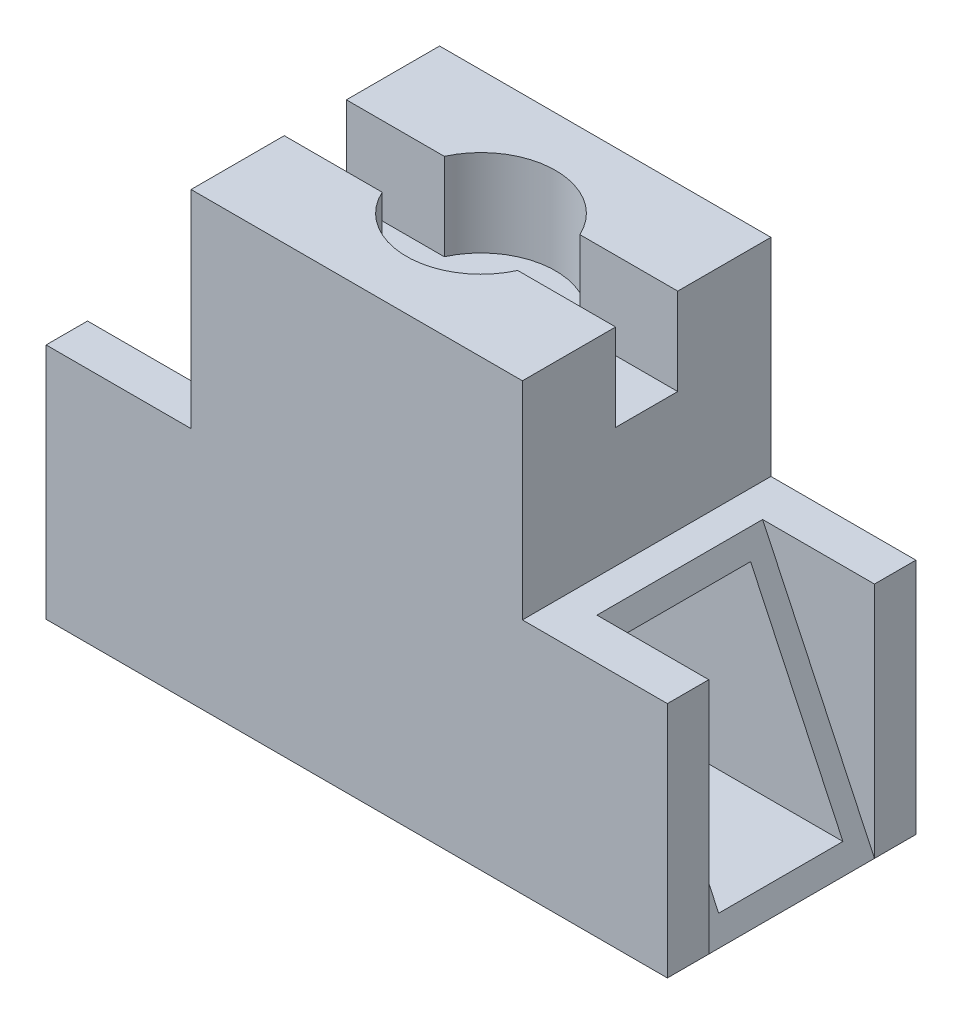
ISO-10303-21;
HEADER;
FILE_DESCRIPTION(('STEP AP214'),'2;1');
FILE_NAME('part.step','',(''),(''),'','','');
FILE_SCHEMA(('AUTOMOTIVE_DESIGN { 1 0 10303 214 1 1 1 1 }'));
ENDSEC;
DATA;
#1=APPLICATION_CONTEXT('core data for automotive mechanical design processes');
#2=APPLICATION_PROTOCOL_DEFINITION('international standard','automotive_design',2000,#1);
#3=PRODUCT_CONTEXT('',#1,'mechanical');
#4=PRODUCT('Part','Part','',(#3));
#5=PRODUCT_RELATED_PRODUCT_CATEGORY('part','',(#4));
#6=PRODUCT_DEFINITION_FORMATION('','',#4);
#7=PRODUCT_DEFINITION_CONTEXT('part definition',#1,'design');
#8=PRODUCT_DEFINITION('design','',#6,#7);
#9=PRODUCT_DEFINITION_SHAPE('','',#8);
#10=(LENGTH_UNIT() NAMED_UNIT(*) SI_UNIT(.MILLI.,.METRE.));
#11=(NAMED_UNIT(*) PLANE_ANGLE_UNIT() SI_UNIT($,.RADIAN.));
#12=(NAMED_UNIT(*) SI_UNIT($,.STERADIAN.) SOLID_ANGLE_UNIT());
#13=UNCERTAINTY_MEASURE_WITH_UNIT(LENGTH_MEASURE(1.E-05),#10,'distance_accuracy_value','');
#14=(GEOMETRIC_REPRESENTATION_CONTEXT(3) GLOBAL_UNCERTAINTY_ASSIGNED_CONTEXT((#13)) GLOBAL_UNIT_ASSIGNED_CONTEXT((#10,
#11,#12)) REPRESENTATION_CONTEXT('',''));
#15=CARTESIAN_POINT('',(0.,0.,0.));
#16=DIRECTION('',(0.,0.,1.));
#17=DIRECTION('',(1.,0.,0.));
#18=AXIS2_PLACEMENT_3D('',#15,#16,#17);
#19=CARTESIAN_POINT('',(75.,28.6870588235294,-60.));
#20=DIRECTION('',(1.,0.,0.));
#21=DIRECTION('',(0.,0.,-1.));
#22=AXIS2_PLACEMENT_3D('',#19,#20,#21);
#23=PLANE('',#22);
#24=DIRECTION('',(0.,0.,1.));
#25=VECTOR('',#24,1.);
#26=CARTESIAN_POINT('',(75.,-28.6870588235294,-60.));
#27=LINE('',#26,#25);
#28=CARTESIAN_POINT('',(75.,-28.6870588235294,-10.));
#29=VERTEX_POINT('',#28);
#30=CARTESIAN_POINT('',(75.,-28.6870588235294,0.));
#31=VERTEX_POINT('',#30);
#32=EDGE_CURVE('E257',#29,#31,#27,.T.);
#33=ORIENTED_EDGE('',*,*,#32,.F.);
#34=DIRECTION('',(0.,1.,0.));
#35=VECTOR('',#34,1.);
#36=CARTESIAN_POINT('',(75.,-28.6870588235294,-10.));
#37=LINE('',#36,#35);
#38=CARTESIAN_POINT('',(75.,28.6870588235294,-10.));
#39=VERTEX_POINT('',#38);
#40=EDGE_CURVE('E399',#29,#39,#37,.T.);
#41=ORIENTED_EDGE('',*,*,#40,.T.);
#42=DIRECTION('',(0.,0.,1.));
#43=VECTOR('',#42,1.);
#44=CARTESIAN_POINT('',(75.,28.6870588235294,-60.));
#45=LINE('',#44,#43);
#46=CARTESIAN_POINT('',(75.,28.6870588235294,0.));
#47=VERTEX_POINT('',#46);
#48=EDGE_CURVE('E255',#39,#47,#45,.T.);
#49=ORIENTED_EDGE('',*,*,#48,.T.);
#50=DIRECTION('',(0.,1.,0.));
#51=VECTOR('',#50,1.);
#52=CARTESIAN_POINT('',(75.,28.6870588235294,0.));
#53=LINE('',#52,#51);
#54=EDGE_CURVE('E286',#31,#47,#53,.T.);
#55=ORIENTED_EDGE('',*,*,#54,.F.);
#56=EDGE_LOOP('',(#33,#41,#49,#55));
#57=FACE_BOUND('',#56,.T.);
#58=ADVANCED_FACE('F39',(#57),#23,.T.);
#59=CARTESIAN_POINT('',(-75.,28.6870588235294,-60.));
#60=DIRECTION('',(-1.,0.,0.));
#61=DIRECTION('',(0.,0.,1.));
#62=AXIS2_PLACEMENT_3D('',#59,#60,#61);
#63=PLANE('',#62);
#64=DIRECTION('',(0.,0.,1.));
#65=VECTOR('',#64,1.);
#66=CARTESIAN_POINT('',(-75.,28.6870588235294,-60.));
#67=LINE('',#66,#65);
#68=CARTESIAN_POINT('',(-75.,28.6870588235294,-10.));
#69=VERTEX_POINT('',#68);
#70=CARTESIAN_POINT('',(-75.,28.6870588235294,0.));
#71=VERTEX_POINT('',#70);
#72=EDGE_CURVE('E232',#69,#71,#67,.T.);
#73=ORIENTED_EDGE('',*,*,#72,.F.);
#74=DIRECTION('',(0.,-1.,0.));
#75=VECTOR('',#74,1.);
#76=CARTESIAN_POINT('',(-75.,-28.6870588235294,-10.));
#77=LINE('',#76,#75);
#78=CARTESIAN_POINT('',(-75.,-28.6870588235294,-10.));
#79=VERTEX_POINT('',#78);
#80=EDGE_CURVE('E417',#69,#79,#77,.T.);
#81=ORIENTED_EDGE('',*,*,#80,.T.);
#82=DIRECTION('',(0.,0.,1.));
#83=VECTOR('',#82,1.);
#84=CARTESIAN_POINT('',(-75.,-28.6870588235294,-60.));
#85=LINE('',#84,#83);
#86=CARTESIAN_POINT('',(-75.,-28.6870588235294,0.));
#87=VERTEX_POINT('',#86);
#88=EDGE_CURVE('E233',#79,#87,#85,.T.);
#89=ORIENTED_EDGE('',*,*,#88,.T.);
#90=DIRECTION('',(0.,-1.,0.));
#91=VECTOR('',#90,1.);
#92=CARTESIAN_POINT('',(-75.,28.6870588235294,0.));
#93=LINE('',#92,#91);
#94=EDGE_CURVE('E267',#71,#87,#93,.T.);
#95=ORIENTED_EDGE('',*,*,#94,.F.);
#96=EDGE_LOOP('',(#73,#81,#89,#95));
#97=FACE_BOUND('',#96,.T.);
#98=ADVANCED_FACE('F430',(#97),#63,.T.);
#99=CARTESIAN_POINT('',(-75.,28.6870588235294,-60.));
#100=DIRECTION('',(0.,1.,0.));
#101=DIRECTION('',(-1.,0.,0.));
#102=AXIS2_PLACEMENT_3D('',#99,#100,#101);
#103=PLANE('',#102);
#104=DIRECTION('',(0.,0.,1.));
#105=VECTOR('',#104,1.);
#106=CARTESIAN_POINT('',(-48.,28.6870588235294,-50.));
#107=LINE('',#106,#105);
#108=CARTESIAN_POINT('',(-48.,28.6870588235294,-50.));
#109=VERTEX_POINT('',#108);
#110=CARTESIAN_POINT('',(-48.,28.6870588235294,-10.));
#111=VERTEX_POINT('',#110);
#112=EDGE_CURVE('E392',#109,#111,#107,.T.);
#113=ORIENTED_EDGE('',*,*,#112,.T.);
#114=DIRECTION('',(-1.,0.,0.));
#115=VECTOR('',#114,1.);
#116=CARTESIAN_POINT('',(-75.,28.6870588235294,-10.));
#117=LINE('',#116,#115);
#118=EDGE_CURVE('E403',#111,#69,#117,.T.);
#119=ORIENTED_EDGE('',*,*,#118,.T.);
#120=ORIENTED_EDGE('',*,*,#72,.T.);
#121=DIRECTION('',(-1.,0.,0.));
#122=VECTOR('',#121,1.);
#123=CARTESIAN_POINT('',(-75.,28.6870588235294,0.));
#124=LINE('',#123,#122);
#125=CARTESIAN_POINT('',(-40.,28.6870588235294,0.));
#126=VERTEX_POINT('',#125);
#127=EDGE_CURVE('E275',#126,#71,#124,.T.);
#128=ORIENTED_EDGE('',*,*,#127,.F.);
#129=DIRECTION('',(0.,0.,1.));
#130=VECTOR('',#129,1.);
#131=CARTESIAN_POINT('',(-40.,28.6870588235294,-60.));
#132=LINE('',#131,#130);
#133=CARTESIAN_POINT('',(-40.,28.6870588235294,-60.));
#134=VERTEX_POINT('',#133);
#135=EDGE_CURVE('E236',#134,#126,#132,.T.);
#136=ORIENTED_EDGE('',*,*,#135,.F.);
#137=DIRECTION('',(-1.,0.,0.));
#138=VECTOR('',#137,1.);
#139=CARTESIAN_POINT('',(-75.,28.6870588235294,-60.));
#140=LINE('',#139,#138);
#141=CARTESIAN_POINT('',(-75.,28.6870588235294,-60.));
#142=VERTEX_POINT('',#141);
#143=EDGE_CURVE('E235',#134,#142,#140,.T.);
#144=ORIENTED_EDGE('',*,*,#143,.T.);
#145=CARTESIAN_POINT('',(-75.,28.6870588235294,-50.));
#146=VERTEX_POINT('',#145);
#147=EDGE_CURVE('E228',#142,#146,#67,.T.);
#148=ORIENTED_EDGE('',*,*,#147,.T.);
#149=DIRECTION('',(-1.,0.,0.));
#150=VECTOR('',#149,1.);
#151=CARTESIAN_POINT('',(-75.,28.6870588235294,-50.));
#152=LINE('',#151,#150);
#153=EDGE_CURVE('E215',#109,#146,#152,.T.);
#154=ORIENTED_EDGE('',*,*,#153,.F.);
#155=EDGE_LOOP('',(#113,#119,#120,#128,#136,#144,#148,#154));
#156=FACE_BOUND('',#155,.T.);
#157=ADVANCED_FACE('F234',(#156),#103,.T.);
#158=CARTESIAN_POINT('',(40.,28.6870588235294,-60.));
#159=DIRECTION('',(0.,1.,0.));
#160=DIRECTION('',(-1.,0.,0.));
#161=AXIS2_PLACEMENT_3D('',#158,#159,#160);
#162=PLANE('',#161);
#163=ORIENTED_EDGE('',*,*,#48,.F.);
#164=DIRECTION('',(-1.,0.,0.));
#165=VECTOR('',#164,1.);
#166=CARTESIAN_POINT('',(75.,28.6870588235294,-10.));
#167=LINE('',#166,#165);
#168=CARTESIAN_POINT('',(48.,28.6870588235294,-10.));
#169=VERTEX_POINT('',#168);
#170=EDGE_CURVE('E405',#39,#169,#167,.T.);
#171=ORIENTED_EDGE('',*,*,#170,.T.);
#172=DIRECTION('',(0.,0.,1.));
#173=VECTOR('',#172,1.);
#174=CARTESIAN_POINT('',(48.,28.6870588235294,-50.));
#175=LINE('',#174,#173);
#176=CARTESIAN_POINT('',(48.,28.6870588235294,-50.));
#177=VERTEX_POINT('',#176);
#178=EDGE_CURVE('E402',#177,#169,#175,.T.);
#179=ORIENTED_EDGE('',*,*,#178,.F.);
#180=DIRECTION('',(-1.,0.,0.));
#181=VECTOR('',#180,1.);
#182=CARTESIAN_POINT('',(75.,28.6870588235294,-50.));
#183=LINE('',#182,#181);
#184=CARTESIAN_POINT('',(75.,28.6870588235294,-50.));
#185=VERTEX_POINT('',#184);
#186=EDGE_CURVE('E65',#185,#177,#183,.T.);
#187=ORIENTED_EDGE('',*,*,#186,.F.);
#188=CARTESIAN_POINT('',(75.,28.6870588235294,-60.));
#189=VERTEX_POINT('',#188);
#190=EDGE_CURVE('E252',#189,#185,#45,.T.);
#191=ORIENTED_EDGE('',*,*,#190,.F.);
#192=DIRECTION('',(-1.,0.,0.));
#193=VECTOR('',#192,1.);
#194=CARTESIAN_POINT('',(40.,28.6870588235294,-60.));
#195=LINE('',#194,#193);
#196=CARTESIAN_POINT('',(40.,28.6870588235294,-60.));
#197=VERTEX_POINT('',#196);
#198=EDGE_CURVE('E302',#189,#197,#195,.T.);
#199=ORIENTED_EDGE('',*,*,#198,.T.);
#200=DIRECTION('',(0.,0.,1.));
#201=VECTOR('',#200,1.);
#202=CARTESIAN_POINT('',(40.,28.6870588235294,-60.));
#203=LINE('',#202,#201);
#204=CARTESIAN_POINT('',(40.,28.6870588235294,0.));
#205=VERTEX_POINT('',#204);
#206=EDGE_CURVE('E247',#197,#205,#203,.T.);
#207=ORIENTED_EDGE('',*,*,#206,.T.);
#208=DIRECTION('',(-1.,0.,0.));
#209=VECTOR('',#208,1.);
#210=CARTESIAN_POINT('',(40.,28.6870588235294,0.));
#211=LINE('',#210,#209);
#212=EDGE_CURVE('E282',#47,#205,#211,.T.);
#213=ORIENTED_EDGE('',*,*,#212,.F.);
#214=EDGE_LOOP('',(#163,#171,#179,#187,#191,#199,#207,#213));
#215=FACE_BOUND('',#214,.T.);
#216=ADVANCED_FACE('F460',(#215),#162,.T.);
#217=CARTESIAN_POINT('',(-40.,78.6870588235294,-60.));
#218=DIRECTION('',(-1.,0.,0.));
#219=DIRECTION('',(0.,-1.,0.));
#220=AXIS2_PLACEMENT_3D('',#217,#218,#219);
#221=PLANE('',#220);
#222=DIRECTION('',(0.,0.,1.));
#223=VECTOR('',#222,1.);
#224=CARTESIAN_POINT('',(-40.,57.6870588235294,-37.5));
#225=LINE('',#224,#223);
#226=CARTESIAN_POINT('',(-40.,57.6870588235294,-37.5));
#227=VERTEX_POINT('',#226);
#228=CARTESIAN_POINT('',(-40.,57.6870588235294,-22.5));
#229=VERTEX_POINT('',#228);
#230=EDGE_CURVE('E329',#227,#229,#225,.T.);
#231=ORIENTED_EDGE('',*,*,#230,.F.);
#232=DIRECTION('',(0.,1.,0.));
#233=VECTOR('',#232,1.);
#234=CARTESIAN_POINT('',(-40.,57.6870588235294,-37.5));
#235=LINE('',#234,#233);
#236=CARTESIAN_POINT('',(-40.,78.6870588235294,-37.5));
#237=VERTEX_POINT('',#236);
#238=EDGE_CURVE('E287',#227,#237,#235,.T.);
#239=ORIENTED_EDGE('',*,*,#238,.T.);
#240=DIRECTION('',(0.,0.,1.));
#241=VECTOR('',#240,1.);
#242=CARTESIAN_POINT('',(-40.,78.6870588235294,-60.));
#243=LINE('',#242,#241);
#244=CARTESIAN_POINT('',(-40.,78.6870588235294,-60.));
#245=VERTEX_POINT('',#244);
#246=EDGE_CURVE('E245',#245,#237,#243,.T.);
#247=ORIENTED_EDGE('',*,*,#246,.F.);
#248=DIRECTION('',(0.,-1.,0.));
#249=VECTOR('',#248,1.);
#250=CARTESIAN_POINT('',(-40.,78.6870588235294,-60.));
#251=LINE('',#250,#249);
#252=EDGE_CURVE('E298',#245,#134,#251,.T.);
#253=ORIENTED_EDGE('',*,*,#252,.T.);
#254=ORIENTED_EDGE('',*,*,#135,.T.);
#255=DIRECTION('',(0.,-1.,0.));
#256=VECTOR('',#255,1.);
#257=CARTESIAN_POINT('',(-40.,78.6870588235294,0.));
#258=LINE('',#257,#256);
#259=CARTESIAN_POINT('',(-40.,78.6870588235294,0.));
#260=VERTEX_POINT('',#259);
#261=EDGE_CURVE('E274',#260,#126,#258,.T.);
#262=ORIENTED_EDGE('',*,*,#261,.F.);
#263=CARTESIAN_POINT('',(-40.,78.6870588235294,-22.5));
#264=VERTEX_POINT('',#263);
#265=EDGE_CURVE('E244',#264,#260,#243,.T.);
#266=ORIENTED_EDGE('',*,*,#265,.F.);
#267=DIRECTION('',(0.,1.,0.));
#268=VECTOR('',#267,1.);
#269=CARTESIAN_POINT('',(-40.,57.6870588235294,-22.5));
#270=LINE('',#269,#268);
#271=EDGE_CURVE('E309',#229,#264,#270,.T.);
#272=ORIENTED_EDGE('',*,*,#271,.F.);
#273=EDGE_LOOP('',(#231,#239,#247,#253,#254,#262,#266,#272));
#274=FACE_BOUND('',#273,.T.);
#275=ADVANCED_FACE('F442',(#274),#221,.T.);
#276=CARTESIAN_POINT('',(-40.,78.6870588235294,-60.));
#277=DIRECTION('',(0.,1.,0.));
#278=DIRECTION('',(-1.,0.,0.));
#279=AXIS2_PLACEMENT_3D('',#276,#277,#278);
#280=PLANE('',#279);
#281=DIRECTION('',(1.,0.,0.));
#282=VECTOR('',#281,1.);
#283=CARTESIAN_POINT('',(-40.,78.6870588235294,-22.5));
#284=LINE('',#283,#282);
#285=CARTESIAN_POINT('',(-16.3630681719536,78.6870588235294,-22.5));
#286=VERTEX_POINT('',#285);
#287=EDGE_CURVE('E341',#264,#286,#284,.T.);
#288=ORIENTED_EDGE('',*,*,#287,.F.);
#289=ORIENTED_EDGE('',*,*,#265,.T.);
#290=DIRECTION('',(-1.,0.,0.));
#291=VECTOR('',#290,1.);
#292=CARTESIAN_POINT('',(-40.,78.6870588235294,0.));
#293=LINE('',#292,#291);
#294=CARTESIAN_POINT('',(40.,78.6870588235294,0.));
#295=VERTEX_POINT('',#294);
#296=EDGE_CURVE('E279',#295,#260,#293,.T.);
#297=ORIENTED_EDGE('',*,*,#296,.F.);
#298=DIRECTION('',(0.,0.,1.));
#299=VECTOR('',#298,1.);
#300=CARTESIAN_POINT('',(40.,78.6870588235294,-60.));
#301=LINE('',#300,#299);
#302=CARTESIAN_POINT('',(40.,78.6870588235294,-22.5));
#303=VERTEX_POINT('',#302);
#304=EDGE_CURVE('E248',#303,#295,#301,.T.);
#305=ORIENTED_EDGE('',*,*,#304,.F.);
#306=DIRECTION('',(1.,0.,0.));
#307=VECTOR('',#306,1.);
#308=CARTESIAN_POINT('',(16.3630681719536,78.6870588235294,-22.5));
#309=LINE('',#308,#307);
#310=CARTESIAN_POINT('',(16.3630681719536,78.6870588235294,-22.5));
#311=VERTEX_POINT('',#310);
#312=EDGE_CURVE('E340',#311,#303,#309,.T.);
#313=ORIENTED_EDGE('',*,*,#312,.F.);
#314=CARTESIAN_POINT('',(0.,78.6870588235294,-30.));
#315=DIRECTION('',(0.,1.,0.));
#316=DIRECTION('',(-1.,0.,0.));
#317=AXIS2_PLACEMENT_3D('',#314,#315,#316);
#318=CIRCLE('',#317,18.);
#319=EDGE_CURVE('E337',#286,#311,#318,.T.);
#320=ORIENTED_EDGE('',*,*,#319,.F.);
#321=EDGE_LOOP('',(#288,#289,#297,#305,#313,#320));
#322=FACE_BOUND('',#321,.T.);
#323=ADVANCED_FACE('F495',(#322),#280,.T.);
#324=CARTESIAN_POINT('',(40.,78.6870588235294,-60.));
#325=DIRECTION('',(1.,0.,0.));
#326=DIRECTION('',(0.,1.,0.));
#327=AXIS2_PLACEMENT_3D('',#324,#325,#326);
#328=PLANE('',#327);
#329=DIRECTION('',(0.,0.,-1.));
#330=VECTOR('',#329,1.);
#331=CARTESIAN_POINT('',(40.,57.6870588235294,-37.5));
#332=LINE('',#331,#330);
#333=CARTESIAN_POINT('',(40.,57.6870588235294,-22.5));
#334=VERTEX_POINT('',#333);
#335=CARTESIAN_POINT('',(40.,57.6870588235294,-37.5));
#336=VERTEX_POINT('',#335);
#337=EDGE_CURVE('E352',#334,#336,#332,.T.);
#338=ORIENTED_EDGE('',*,*,#337,.F.);
#339=DIRECTION('',(0.,1.,0.));
#340=VECTOR('',#339,1.);
#341=CARTESIAN_POINT('',(40.,57.6870588235294,-22.5));
#342=LINE('',#341,#340);
#343=EDGE_CURVE('E320',#334,#303,#342,.T.);
#344=ORIENTED_EDGE('',*,*,#343,.T.);
#345=ORIENTED_EDGE('',*,*,#304,.T.);
#346=DIRECTION('',(0.,1.,0.));
#347=VECTOR('',#346,1.);
#348=CARTESIAN_POINT('',(40.,78.6870588235294,0.));
#349=LINE('',#348,#347);
#350=EDGE_CURVE('E283',#205,#295,#349,.T.);
#351=ORIENTED_EDGE('',*,*,#350,.F.);
#352=ORIENTED_EDGE('',*,*,#206,.F.);
#353=DIRECTION('',(0.,1.,0.));
#354=VECTOR('',#353,1.);
#355=CARTESIAN_POINT('',(40.,78.6870588235294,-60.));
#356=LINE('',#355,#354);
#357=CARTESIAN_POINT('',(40.,78.6870588235294,-60.));
#358=VERTEX_POINT('',#357);
#359=EDGE_CURVE('E301',#197,#358,#356,.T.);
#360=ORIENTED_EDGE('',*,*,#359,.T.);
#361=CARTESIAN_POINT('',(40.,78.6870588235294,-37.5));
#362=VERTEX_POINT('',#361);
#363=EDGE_CURVE('E249',#358,#362,#301,.T.);
#364=ORIENTED_EDGE('',*,*,#363,.T.);
#365=DIRECTION('',(0.,1.,0.));
#366=VECTOR('',#365,1.);
#367=CARTESIAN_POINT('',(40.,57.6870588235294,-37.5));
#368=LINE('',#367,#366);
#369=EDGE_CURVE('E319',#336,#362,#368,.T.);
#370=ORIENTED_EDGE('',*,*,#369,.F.);
#371=EDGE_LOOP('',(#338,#344,#345,#351,#352,#360,#364,#370));
#372=FACE_BOUND('',#371,.T.);
#373=ADVANCED_FACE('F454',(#372),#328,.T.);
#374=DIRECTION('',(0.,1.,0.));
#375=VECTOR('',#374,1.);
#376=CARTESIAN_POINT('',(75.,-28.6870588235294,-50.));
#377=LINE('',#376,#375);
#378=CARTESIAN_POINT('',(75.,-28.6870588235294,-50.));
#379=VERTEX_POINT('',#378);
#380=EDGE_CURVE('E398',#379,#185,#377,.T.);
#381=ORIENTED_EDGE('',*,*,#380,.F.);
#382=CARTESIAN_POINT('',(75.,-28.6870588235294,-60.));
#383=VERTEX_POINT('',#382);
#384=EDGE_CURVE('E254',#383,#379,#27,.T.);
#385=ORIENTED_EDGE('',*,*,#384,.F.);
#386=DIRECTION('',(0.,1.,0.));
#387=VECTOR('',#386,1.);
#388=CARTESIAN_POINT('',(75.,28.6870588235294,-60.));
#389=LINE('',#388,#387);
#390=EDGE_CURVE('E268',#383,#189,#389,.T.);
#391=ORIENTED_EDGE('',*,*,#390,.T.);
#392=ORIENTED_EDGE('',*,*,#190,.T.);
#393=EDGE_LOOP('',(#381,#385,#391,#392));
#394=FACE_BOUND('',#393,.T.);
#395=ADVANCED_FACE('F41',(#394),#23,.T.);
#396=CARTESIAN_POINT('',(-75.,-28.6870588235294,-60.));
#397=DIRECTION('',(0.,-1.,0.));
#398=DIRECTION('',(0.,0.,-1.));
#399=AXIS2_PLACEMENT_3D('',#396,#397,#398);
#400=PLANE('',#399);
#401=DIRECTION('',(1.,0.,0.));
#402=VECTOR('',#401,1.);
#403=CARTESIAN_POINT('',(-75.,-28.6870588235294,0.));
#404=LINE('',#403,#402);
#405=EDGE_CURVE('E264',#87,#31,#404,.T.);
#406=ORIENTED_EDGE('',*,*,#405,.F.);
#407=ORIENTED_EDGE('',*,*,#88,.F.);
#408=DIRECTION('',(0.,0.,1.));
#409=VECTOR('',#408,1.);
#410=CARTESIAN_POINT('',(-75.,-28.6870588235294,-50.));
#411=LINE('',#410,#409);
#412=CARTESIAN_POINT('',(-75.,-28.6870588235294,-50.));
#413=VERTEX_POINT('',#412);
#414=EDGE_CURVE('E415',#413,#79,#411,.T.);
#415=ORIENTED_EDGE('',*,*,#414,.F.);
#416=CARTESIAN_POINT('',(-75.,-28.6870588235294,-60.));
#417=VERTEX_POINT('',#416);
#418=EDGE_CURVE('E226',#417,#413,#85,.T.);
#419=ORIENTED_EDGE('',*,*,#418,.F.);
#420=DIRECTION('',(1.,0.,0.));
#421=VECTOR('',#420,1.);
#422=CARTESIAN_POINT('',(-75.,-28.6870588235294,-60.));
#423=LINE('',#422,#421);
#424=EDGE_CURVE('E292',#417,#383,#423,.T.);
#425=ORIENTED_EDGE('',*,*,#424,.T.);
#426=ORIENTED_EDGE('',*,*,#384,.T.);
#427=DIRECTION('',(0.,0.,1.));
#428=VECTOR('',#427,1.);
#429=CARTESIAN_POINT('',(75.,-28.6870588235294,-50.));
#430=LINE('',#429,#428);
#431=EDGE_CURVE('E409',#379,#29,#430,.T.);
#432=ORIENTED_EDGE('',*,*,#431,.T.);
#433=ORIENTED_EDGE('',*,*,#32,.T.);
#434=EDGE_LOOP('',(#406,#407,#415,#419,#425,#426,#432,#433));
#435=FACE_BOUND('',#434,.T.);
#436=ADVANCED_FACE('F473',(#435),#400,.T.);
#437=DIRECTION('',(0.,-1.,0.));
#438=VECTOR('',#437,1.);
#439=CARTESIAN_POINT('',(-75.,-28.6870588235294,-50.));
#440=LINE('',#439,#438);
#441=EDGE_CURVE('E214',#146,#413,#440,.T.);
#442=ORIENTED_EDGE('',*,*,#441,.F.);
#443=ORIENTED_EDGE('',*,*,#147,.F.);
#444=DIRECTION('',(0.,-1.,0.));
#445=VECTOR('',#444,1.);
#446=CARTESIAN_POINT('',(-75.,28.6870588235294,-60.));
#447=LINE('',#446,#445);
#448=EDGE_CURVE('E291',#142,#417,#447,.T.);
#449=ORIENTED_EDGE('',*,*,#448,.T.);
#450=ORIENTED_EDGE('',*,*,#418,.T.);
#451=EDGE_LOOP('',(#442,#443,#449,#450));
#452=FACE_BOUND('',#451,.T.);
#453=ADVANCED_FACE('F221',(#452),#63,.T.);
#454=DIRECTION('',(-1.,0.,0.));
#455=VECTOR('',#454,1.);
#456=CARTESIAN_POINT('',(16.3630681719536,78.6870588235294,-37.5));
#457=LINE('',#456,#455);
#458=CARTESIAN_POINT('',(16.3630681719536,78.6870588235294,-37.5));
#459=VERTEX_POINT('',#458);
#460=EDGE_CURVE('E331',#362,#459,#457,.T.);
#461=ORIENTED_EDGE('',*,*,#460,.F.);
#462=ORIENTED_EDGE('',*,*,#363,.F.);
#463=DIRECTION('',(-1.,0.,0.));
#464=VECTOR('',#463,1.);
#465=CARTESIAN_POINT('',(-40.,78.6870588235294,-60.));
#466=LINE('',#465,#464);
#467=EDGE_CURVE('E297',#358,#245,#466,.T.);
#468=ORIENTED_EDGE('',*,*,#467,.T.);
#469=ORIENTED_EDGE('',*,*,#246,.T.);
#470=DIRECTION('',(-1.,0.,0.));
#471=VECTOR('',#470,1.);
#472=CARTESIAN_POINT('',(-40.,78.6870588235294,-37.5));
#473=LINE('',#472,#471);
#474=CARTESIAN_POINT('',(-16.3630681719536,78.6870588235294,-37.5));
#475=VERTEX_POINT('',#474);
#476=EDGE_CURVE('E327',#475,#237,#473,.T.);
#477=ORIENTED_EDGE('',*,*,#476,.F.);
#478=CARTESIAN_POINT('',(0.,78.6870588235294,-30.));
#479=DIRECTION('',(0.,1.,0.));
#480=DIRECTION('',(-1.,0.,0.));
#481=AXIS2_PLACEMENT_3D('',#478,#479,#480);
#482=CIRCLE('',#481,18.);
#483=EDGE_CURVE('E332',#459,#475,#482,.T.);
#484=ORIENTED_EDGE('',*,*,#483,.F.);
#485=EDGE_LOOP('',(#461,#462,#468,#469,#477,#484));
#486=FACE_BOUND('',#485,.T.);
#487=ADVANCED_FACE('F443',(#486),#280,.T.);
#488=CARTESIAN_POINT('',(0.,0.,-60.));
#489=DIRECTION('',(0.,0.,1.));
#490=DIRECTION('',(1.,0.,0.));
#491=AXIS2_PLACEMENT_3D('',#488,#489,#490);
#492=PLANE('',#491);
#493=ORIENTED_EDGE('',*,*,#390,.F.);
#494=ORIENTED_EDGE('',*,*,#424,.F.);
#495=ORIENTED_EDGE('',*,*,#448,.F.);
#496=ORIENTED_EDGE('',*,*,#143,.F.);
#497=ORIENTED_EDGE('',*,*,#252,.F.);
#498=ORIENTED_EDGE('',*,*,#467,.F.);
#499=ORIENTED_EDGE('',*,*,#359,.F.);
#500=ORIENTED_EDGE('',*,*,#198,.F.);
#501=EDGE_LOOP('',(#493,#494,#495,#496,#497,#498,#499,#500));
#502=FACE_BOUND('',#501,.T.);
#503=ADVANCED_FACE('F440',(#502),#492,.F.);
#504=CARTESIAN_POINT('',(0.,0.,0.));
#505=DIRECTION('',(0.,0.,1.));
#506=DIRECTION('',(1.,0.,0.));
#507=AXIS2_PLACEMENT_3D('',#504,#505,#506);
#508=PLANE('',#507);
#509=ORIENTED_EDGE('',*,*,#54,.T.);
#510=ORIENTED_EDGE('',*,*,#212,.T.);
#511=ORIENTED_EDGE('',*,*,#350,.T.);
#512=ORIENTED_EDGE('',*,*,#296,.T.);
#513=ORIENTED_EDGE('',*,*,#261,.T.);
#514=ORIENTED_EDGE('',*,*,#127,.T.);
#515=ORIENTED_EDGE('',*,*,#94,.T.);
#516=ORIENTED_EDGE('',*,*,#405,.T.);
#517=EDGE_LOOP('',(#509,#510,#511,#512,#513,#514,#515,#516));
#518=FACE_BOUND('',#517,.T.);
#519=ADVANCED_FACE('F431',(#518),#508,.T.);
#520=CARTESIAN_POINT('',(-40.,57.6870588235294,-37.5));
#521=DIRECTION('',(0.,0.,-1.));
#522=DIRECTION('',(-1.,0.,0.));
#523=AXIS2_PLACEMENT_3D('',#520,#521,#522);
#524=PLANE('',#523);
#525=ORIENTED_EDGE('',*,*,#476,.T.);
#526=ORIENTED_EDGE('',*,*,#238,.F.);
#527=DIRECTION('',(-1.,0.,0.));
#528=VECTOR('',#527,1.);
#529=CARTESIAN_POINT('',(-40.,57.6870588235294,-37.5));
#530=LINE('',#529,#528);
#531=CARTESIAN_POINT('',(-16.3630681719536,57.6870588235294,-37.5));
#532=VERTEX_POINT('',#531);
#533=EDGE_CURVE('E311',#532,#227,#530,.T.);
#534=ORIENTED_EDGE('',*,*,#533,.F.);
#535=DIRECTION('',(0.,1.,0.));
#536=VECTOR('',#535,1.);
#537=CARTESIAN_POINT('',(-16.3630681719536,57.6870588235294,-37.5));
#538=LINE('',#537,#536);
#539=EDGE_CURVE('E322',#532,#475,#538,.T.);
#540=ORIENTED_EDGE('',*,*,#539,.T.);
#541=EDGE_LOOP('',(#525,#526,#534,#540));
#542=FACE_BOUND('',#541,.T.);
#543=ADVANCED_FACE('F545',(#542),#524,.F.);
#544=CARTESIAN_POINT('',(0.,57.6870588235294,-30.));
#545=DIRECTION('',(0.,1.,0.));
#546=DIRECTION('',(-1.,0.,0.));
#547=AXIS2_PLACEMENT_3D('',#544,#545,#546);
#548=CYLINDRICAL_SURFACE('',#547,18.);
#549=ORIENTED_EDGE('',*,*,#483,.T.);
#550=ORIENTED_EDGE('',*,*,#539,.F.);
#551=CARTESIAN_POINT('',(0.,57.6870588235294,-30.));
#552=DIRECTION('',(0.,1.,0.));
#553=DIRECTION('',(-1.,0.,0.));
#554=AXIS2_PLACEMENT_3D('',#551,#552,#553);
#555=CIRCLE('',#554,18.);
#556=CARTESIAN_POINT('',(16.3630681719536,57.6870588235294,-37.5));
#557=VERTEX_POINT('',#556);
#558=EDGE_CURVE('E346',#557,#532,#555,.T.);
#559=ORIENTED_EDGE('',*,*,#558,.F.);
#560=DIRECTION('',(0.,1.,0.));
#561=VECTOR('',#560,1.);
#562=CARTESIAN_POINT('',(16.3630681719536,57.6870588235294,-37.5));
#563=LINE('',#562,#561);
#564=EDGE_CURVE('E325',#557,#459,#563,.T.);
#565=ORIENTED_EDGE('',*,*,#564,.T.);
#566=EDGE_LOOP('',(#549,#550,#559,#565));
#567=FACE_BOUND('',#566,.T.);
#568=ADVANCED_FACE('F567',(#567),#548,.F.);
#569=CARTESIAN_POINT('',(16.3630681719536,57.6870588235294,-37.5));
#570=DIRECTION('',(0.,0.,-1.));
#571=DIRECTION('',(-1.,0.,0.));
#572=AXIS2_PLACEMENT_3D('',#569,#570,#571);
#573=PLANE('',#572);
#574=ORIENTED_EDGE('',*,*,#460,.T.);
#575=ORIENTED_EDGE('',*,*,#564,.F.);
#576=DIRECTION('',(-1.,0.,0.));
#577=VECTOR('',#576,1.);
#578=CARTESIAN_POINT('',(16.3630681719536,57.6870588235294,-37.5));
#579=LINE('',#578,#577);
#580=EDGE_CURVE('E353',#336,#557,#579,.T.);
#581=ORIENTED_EDGE('',*,*,#580,.F.);
#582=ORIENTED_EDGE('',*,*,#369,.T.);
#583=EDGE_LOOP('',(#574,#575,#581,#582));
#584=FACE_BOUND('',#583,.T.);
#585=ADVANCED_FACE('F579',(#584),#573,.F.);
#586=CARTESIAN_POINT('',(16.3630681719536,57.6870588235294,-22.5));
#587=DIRECTION('',(0.,0.,1.));
#588=DIRECTION('',(1.,0.,0.));
#589=AXIS2_PLACEMENT_3D('',#586,#587,#588);
#590=PLANE('',#589);
#591=ORIENTED_EDGE('',*,*,#312,.T.);
#592=ORIENTED_EDGE('',*,*,#343,.F.);
#593=DIRECTION('',(1.,0.,0.));
#594=VECTOR('',#593,1.);
#595=CARTESIAN_POINT('',(16.3630681719536,57.6870588235294,-22.5));
#596=LINE('',#595,#594);
#597=CARTESIAN_POINT('',(16.3630681719536,57.6870588235294,-22.5));
#598=VERTEX_POINT('',#597);
#599=EDGE_CURVE('E356',#598,#334,#596,.T.);
#600=ORIENTED_EDGE('',*,*,#599,.F.);
#601=DIRECTION('',(0.,1.,0.));
#602=VECTOR('',#601,1.);
#603=CARTESIAN_POINT('',(16.3630681719536,57.6870588235294,-22.5));
#604=LINE('',#603,#602);
#605=EDGE_CURVE('E312',#598,#311,#604,.T.);
#606=ORIENTED_EDGE('',*,*,#605,.T.);
#607=EDGE_LOOP('',(#591,#592,#600,#606));
#608=FACE_BOUND('',#607,.T.);
#609=ADVANCED_FACE('F588',(#608),#590,.F.);
#610=CARTESIAN_POINT('',(0.,57.6870588235294,-30.));
#611=DIRECTION('',(0.,1.,0.));
#612=DIRECTION('',(-1.,0.,0.));
#613=AXIS2_PLACEMENT_3D('',#610,#611,#612);
#614=CYLINDRICAL_SURFACE('',#613,18.);
#615=ORIENTED_EDGE('',*,*,#319,.T.);
#616=ORIENTED_EDGE('',*,*,#605,.F.);
#617=CARTESIAN_POINT('',(0.,57.6870588235294,-30.));
#618=DIRECTION('',(0.,1.,0.));
#619=DIRECTION('',(-1.,0.,0.));
#620=AXIS2_PLACEMENT_3D('',#617,#618,#619);
#621=CIRCLE('',#620,18.);
#622=CARTESIAN_POINT('',(-16.3630681719536,57.6870588235294,-22.5));
#623=VERTEX_POINT('',#622);
#624=EDGE_CURVE('E358',#623,#598,#621,.T.);
#625=ORIENTED_EDGE('',*,*,#624,.F.);
#626=DIRECTION('',(0.,1.,0.));
#627=VECTOR('',#626,1.);
#628=CARTESIAN_POINT('',(-16.3630681719536,57.6870588235294,-22.5));
#629=LINE('',#628,#627);
#630=EDGE_CURVE('E315',#623,#286,#629,.T.);
#631=ORIENTED_EDGE('',*,*,#630,.T.);
#632=EDGE_LOOP('',(#615,#616,#625,#631));
#633=FACE_BOUND('',#632,.T.);
#634=ADVANCED_FACE('F596',(#633),#614,.F.);
#635=CARTESIAN_POINT('',(-40.,57.6870588235294,-22.5));
#636=DIRECTION('',(0.,0.,1.));
#637=DIRECTION('',(1.,0.,0.));
#638=AXIS2_PLACEMENT_3D('',#635,#636,#637);
#639=PLANE('',#638);
#640=ORIENTED_EDGE('',*,*,#287,.T.);
#641=ORIENTED_EDGE('',*,*,#630,.F.);
#642=DIRECTION('',(1.,0.,0.));
#643=VECTOR('',#642,1.);
#644=CARTESIAN_POINT('',(-40.,57.6870588235294,-22.5));
#645=LINE('',#644,#643);
#646=EDGE_CURVE('E362',#229,#623,#645,.T.);
#647=ORIENTED_EDGE('',*,*,#646,.F.);
#648=ORIENTED_EDGE('',*,*,#271,.T.);
#649=EDGE_LOOP('',(#640,#641,#647,#648));
#650=FACE_BOUND('',#649,.T.);
#651=ADVANCED_FACE('F607',(#650),#639,.F.);
#652=CARTESIAN_POINT('',(0.,57.6870588235294,-30.));
#653=DIRECTION('',(0.,1.,0.));
#654=DIRECTION('',(-1.,0.,0.));
#655=AXIS2_PLACEMENT_3D('',#652,#653,#654);
#656=PLANE('',#655);
#657=ORIENTED_EDGE('',*,*,#230,.T.);
#658=ORIENTED_EDGE('',*,*,#646,.T.);
#659=ORIENTED_EDGE('',*,*,#624,.T.);
#660=ORIENTED_EDGE('',*,*,#599,.T.);
#661=ORIENTED_EDGE('',*,*,#337,.T.);
#662=ORIENTED_EDGE('',*,*,#580,.T.);
#663=ORIENTED_EDGE('',*,*,#558,.T.);
#664=ORIENTED_EDGE('',*,*,#533,.T.);
#665=EDGE_LOOP('',(#657,#658,#659,#660,#661,#662,#663,#664));
#666=FACE_BOUND('',#665,.T.);
#667=ADVANCED_FACE('F619',(#666),#656,.T.);
#668=CARTESIAN_POINT('',(48.,28.6870588235294,-50.));
#669=DIRECTION('',(-0.904816179332122,-0.42580239738501,0.));
#670=DIRECTION('',(0.42580239738501,-0.904816179332122,0.));
#671=AXIS2_PLACEMENT_3D('',#668,#669,#670);
#672=PLANE('',#671);
#673=DIRECTION('',(0.42580239738501,-0.904816179332121,0.));
#674=VECTOR('',#673,1.);
#675=CARTESIAN_POINT('',(48.,28.6870588235294,-10.));
#676=LINE('',#675,#674);
#677=EDGE_CURVE('E408',#169,#29,#676,.T.);
#678=ORIENTED_EDGE('',*,*,#677,.T.);
#679=ORIENTED_EDGE('',*,*,#431,.F.);
#680=DIRECTION('',(0.42580239738501,-0.904816179332121,0.));
#681=VECTOR('',#680,1.);
#682=CARTESIAN_POINT('',(48.,28.6870588235294,-50.));
#683=LINE('',#682,#681);
#684=EDGE_CURVE('E396',#177,#379,#683,.T.);
#685=ORIENTED_EDGE('',*,*,#684,.F.);
#686=ORIENTED_EDGE('',*,*,#178,.T.);
#687=EDGE_LOOP('',(#678,#679,#685,#686));
#688=FACE_BOUND('',#687,.T.);
#689=DIRECTION('',(-0.42580239738501,0.904816179332122,0.));
#690=VECTOR('',#689,1.);
#691=CARTESIAN_POINT('',(54.82167189547,14.1912289761097,-14.7406029561998));
#692=LINE('',#691,#690);
#693=CARTESIAN_POINT('',(72.6470226377953,-23.6870588235294,-14.7406029561998));
#694=VERTEX_POINT('',#693);
#695=CARTESIAN_POINT('',(50.3529773622047,23.6870588235294,-14.7406029561998));
#696=VERTEX_POINT('',#695);
#697=EDGE_CURVE('E50',#694,#696,#692,.T.);
#698=ORIENTED_EDGE('',*,*,#697,.T.);
#699=DIRECTION('',(0.,0.,-1.));
#700=VECTOR('',#699,1.);
#701=CARTESIAN_POINT('',(50.3529773622047,23.6870588235294,-44.7406029561998));
#702=LINE('',#701,#700);
#703=CARTESIAN_POINT('',(50.3529773622047,23.6870588235294,-44.7406029561998));
#704=VERTEX_POINT('',#703);
#705=EDGE_CURVE('E395',#696,#704,#702,.T.);
#706=ORIENTED_EDGE('',*,*,#705,.T.);
#707=DIRECTION('',(-0.42580239738501,0.904816179332122,0.));
#708=VECTOR('',#707,1.);
#709=CARTESIAN_POINT('',(54.82167189547,14.1912289761097,-44.7406029561998));
#710=LINE('',#709,#708);
#711=CARTESIAN_POINT('',(72.6470226377952,-23.6870588235294,-44.7406029561998));
#712=VERTEX_POINT('',#711);
#713=EDGE_CURVE('E386',#712,#704,#710,.T.);
#714=ORIENTED_EDGE('',*,*,#713,.F.);
#715=DIRECTION('',(0.,0.,-1.));
#716=VECTOR('',#715,1.);
#717=CARTESIAN_POINT('',(72.6470226377952,-23.6870588235294,-44.7406029561998));
#718=LINE('',#717,#716);
#719=EDGE_CURVE('E387',#694,#712,#718,.T.);
#720=ORIENTED_EDGE('',*,*,#719,.F.);
#721=EDGE_LOOP('',(#698,#706,#714,#720));
#722=FACE_BOUND('',#721,.T.);
#723=ADVANCED_FACE('F462',(#688,#722),#672,.F.);
#724=CARTESIAN_POINT('',(0.,0.,-50.));
#725=DIRECTION('',(0.,0.,-1.));
#726=DIRECTION('',(-1.,0.,0.));
#727=AXIS2_PLACEMENT_3D('',#724,#725,#726);
#728=PLANE('',#727);
#729=ORIENTED_EDGE('',*,*,#186,.T.);
#730=ORIENTED_EDGE('',*,*,#684,.T.);
#731=ORIENTED_EDGE('',*,*,#380,.T.);
#732=EDGE_LOOP('',(#729,#730,#731));
#733=FACE_BOUND('',#732,.T.);
#734=ADVANCED_FACE('F458',(#733),#728,.F.);
#735=CARTESIAN_POINT('',(0.,0.,-10.));
#736=DIRECTION('',(0.,0.,-1.));
#737=DIRECTION('',(-1.,0.,0.));
#738=AXIS2_PLACEMENT_3D('',#735,#736,#737);
#739=PLANE('',#738);
#740=ORIENTED_EDGE('',*,*,#170,.F.);
#741=ORIENTED_EDGE('',*,*,#40,.F.);
#742=ORIENTED_EDGE('',*,*,#677,.F.);
#743=EDGE_LOOP('',(#740,#741,#742));
#744=FACE_BOUND('',#743,.T.);
#745=ADVANCED_FACE('F466',(#744),#739,.T.);
#746=CARTESIAN_POINT('',(-48.,28.6870588235294,-50.));
#747=DIRECTION('',(0.904816179332121,-0.42580239738501,0.));
#748=DIRECTION('',(0.425802397385011,0.904816179332122,0.));
#749=AXIS2_PLACEMENT_3D('',#746,#747,#748);
#750=PLANE('',#749);
#751=DIRECTION('',(0.42580239738501,0.904816179332121,0.));
#752=VECTOR('',#751,1.);
#753=CARTESIAN_POINT('',(-48.,28.6870588235294,-10.));
#754=LINE('',#753,#752);
#755=EDGE_CURVE('E53',#79,#111,#754,.T.);
#756=ORIENTED_EDGE('',*,*,#755,.T.);
#757=ORIENTED_EDGE('',*,*,#112,.F.);
#758=DIRECTION('',(0.42580239738501,0.904816179332121,0.));
#759=VECTOR('',#758,1.);
#760=CARTESIAN_POINT('',(-48.,28.6870588235294,-50.));
#761=LINE('',#760,#759);
#762=EDGE_CURVE('E220',#413,#109,#761,.T.);
#763=ORIENTED_EDGE('',*,*,#762,.F.);
#764=ORIENTED_EDGE('',*,*,#414,.T.);
#765=EDGE_LOOP('',(#756,#757,#763,#764));
#766=FACE_BOUND('',#765,.T.);
#767=DIRECTION('',(-0.425802397385011,-0.904816179332122,0.));
#768=VECTOR('',#767,1.);
#769=CARTESIAN_POINT('',(-27.6255196526467,71.9821637289642,-44.7406029561998));
#770=LINE('',#769,#768);
#771=CARTESIAN_POINT('',(-50.3529773622047,23.6870588235294,-44.7406029561998));
#772=VERTEX_POINT('',#771);
#773=CARTESIAN_POINT('',(-72.6470226377953,-23.6870588235294,-44.7406029561998));
#774=VERTEX_POINT('',#773);
#775=EDGE_CURVE('E381',#772,#774,#770,.T.);
#776=ORIENTED_EDGE('',*,*,#775,.F.);
#777=DIRECTION('',(0.,0.,1.));
#778=VECTOR('',#777,1.);
#779=CARTESIAN_POINT('',(-50.3529773622047,23.6870588235294,-44.7406029561998));
#780=LINE('',#779,#778);
#781=CARTESIAN_POINT('',(-50.3529773622047,23.6870588235294,-14.7406029561998));
#782=VERTEX_POINT('',#781);
#783=EDGE_CURVE('E383',#772,#782,#780,.T.);
#784=ORIENTED_EDGE('',*,*,#783,.T.);
#785=DIRECTION('',(-0.425802397385011,-0.904816179332122,0.));
#786=VECTOR('',#785,1.);
#787=CARTESIAN_POINT('',(-27.6255196526467,71.9821637289642,-14.7406029561998));
#788=LINE('',#787,#786);
#789=CARTESIAN_POINT('',(-72.6470226377953,-23.6870588235294,-14.7406029561998));
#790=VERTEX_POINT('',#789);
#791=EDGE_CURVE('E11',#782,#790,#788,.T.);
#792=ORIENTED_EDGE('',*,*,#791,.T.);
#793=DIRECTION('',(0.,0.,1.));
#794=VECTOR('',#793,1.);
#795=CARTESIAN_POINT('',(-72.6470226377953,-23.6870588235294,-44.7406029561998));
#796=LINE('',#795,#794);
#797=EDGE_CURVE('E371',#774,#790,#796,.T.);
#798=ORIENTED_EDGE('',*,*,#797,.F.);
#799=EDGE_LOOP('',(#776,#784,#792,#798));
#800=FACE_BOUND('',#799,.T.);
#801=ADVANCED_FACE('F702',(#766,#800),#750,.F.);
#802=CARTESIAN_POINT('',(0.,0.,-50.));
#803=DIRECTION('',(0.,0.,1.));
#804=DIRECTION('',(1.,0.,0.));
#805=AXIS2_PLACEMENT_3D('',#802,#803,#804);
#806=PLANE('',#805);
#807=ORIENTED_EDGE('',*,*,#153,.T.);
#808=ORIENTED_EDGE('',*,*,#441,.T.);
#809=ORIENTED_EDGE('',*,*,#762,.T.);
#810=EDGE_LOOP('',(#807,#808,#809));
#811=FACE_BOUND('',#810,.T.);
#812=ADVANCED_FACE('F212',(#811),#806,.T.);
#813=CARTESIAN_POINT('',(0.,0.,-10.));
#814=DIRECTION('',(0.,0.,1.));
#815=DIRECTION('',(1.,0.,0.));
#816=AXIS2_PLACEMENT_3D('',#813,#814,#815);
#817=PLANE('',#816);
#818=ORIENTED_EDGE('',*,*,#118,.F.);
#819=ORIENTED_EDGE('',*,*,#755,.F.);
#820=ORIENTED_EDGE('',*,*,#80,.F.);
#821=EDGE_LOOP('',(#818,#819,#820));
#822=FACE_BOUND('',#821,.T.);
#823=ADVANCED_FACE('F664',(#822),#817,.F.);
#824=CARTESIAN_POINT('',(75.,23.6870588235294,-14.7406029561998));
#825=DIRECTION('',(0.,0.,-1.));
#826=DIRECTION('',(0.,1.,0.));
#827=AXIS2_PLACEMENT_3D('',#824,#825,#826);
#828=PLANE('',#827);
#829=ORIENTED_EDGE('',*,*,#791,.F.);
#830=DIRECTION('',(-1.,0.,0.));
#831=VECTOR('',#830,1.);
#832=CARTESIAN_POINT('',(75.,23.6870588235294,-14.7406029561998));
#833=LINE('',#832,#831);
#834=EDGE_CURVE('E367',#696,#782,#833,.T.);
#835=ORIENTED_EDGE('',*,*,#834,.F.);
#836=ORIENTED_EDGE('',*,*,#697,.F.);
#837=DIRECTION('',(-1.,0.,0.));
#838=VECTOR('',#837,1.);
#839=CARTESIAN_POINT('',(75.,-23.6870588235294,-14.7406029561998));
#840=LINE('',#839,#838);
#841=EDGE_CURVE('E370',#694,#790,#840,.T.);
#842=ORIENTED_EDGE('',*,*,#841,.T.);
#843=EDGE_LOOP('',(#829,#835,#836,#842));
#844=FACE_BOUND('',#843,.T.);
#845=ADVANCED_FACE('F654',(#844),#828,.T.);
#846=CARTESIAN_POINT('',(75.,23.6870588235294,-44.7406029561998));
#847=DIRECTION('',(0.,-1.,0.));
#848=DIRECTION('',(0.,0.,-1.));
#849=AXIS2_PLACEMENT_3D('',#846,#847,#848);
#850=PLANE('',#849);
#851=ORIENTED_EDGE('',*,*,#783,.F.);
#852=DIRECTION('',(-1.,0.,0.));
#853=VECTOR('',#852,1.);
#854=CARTESIAN_POINT('',(75.,23.6870588235294,-44.7406029561998));
#855=LINE('',#854,#853);
#856=EDGE_CURVE('E372',#704,#772,#855,.T.);
#857=ORIENTED_EDGE('',*,*,#856,.F.);
#858=ORIENTED_EDGE('',*,*,#705,.F.);
#859=ORIENTED_EDGE('',*,*,#834,.T.);
#860=EDGE_LOOP('',(#851,#857,#858,#859));
#861=FACE_BOUND('',#860,.T.);
#862=ADVANCED_FACE('F642',(#861),#850,.T.);
#863=CARTESIAN_POINT('',(75.,23.6870588235294,-44.7406029561998));
#864=DIRECTION('',(0.,0.,-1.));
#865=DIRECTION('',(0.,1.,0.));
#866=AXIS2_PLACEMENT_3D('',#863,#864,#865);
#867=PLANE('',#866);
#868=ORIENTED_EDGE('',*,*,#856,.T.);
#869=ORIENTED_EDGE('',*,*,#775,.T.);
#870=DIRECTION('',(-1.,0.,0.));
#871=VECTOR('',#870,1.);
#872=CARTESIAN_POINT('',(75.,-23.6870588235294,-44.7406029561998));
#873=LINE('',#872,#871);
#874=EDGE_CURVE('E342',#712,#774,#873,.T.);
#875=ORIENTED_EDGE('',*,*,#874,.F.);
#876=ORIENTED_EDGE('',*,*,#713,.T.);
#877=EDGE_LOOP('',(#868,#869,#875,#876));
#878=FACE_BOUND('',#877,.T.);
#879=ADVANCED_FACE('F632',(#878),#867,.F.);
#880=CARTESIAN_POINT('',(75.,-23.6870588235294,-44.7406029561998));
#881=DIRECTION('',(0.,-1.,0.));
#882=DIRECTION('',(0.,0.,-1.));
#883=AXIS2_PLACEMENT_3D('',#880,#881,#882);
#884=PLANE('',#883);
#885=ORIENTED_EDGE('',*,*,#874,.T.);
#886=ORIENTED_EDGE('',*,*,#797,.T.);
#887=ORIENTED_EDGE('',*,*,#841,.F.);
#888=ORIENTED_EDGE('',*,*,#719,.T.);
#889=EDGE_LOOP('',(#885,#886,#887,#888));
#890=FACE_BOUND('',#889,.T.);
#891=ADVANCED_FACE('F629',(#890),#884,.F.);
#892=CLOSED_SHELL('',(#58,#98,#157,#216,#275,#323,#373,#395,#436,#453,#487,#503,#519,#543,#568,
#585,#609,#634,#651,#667,#723,#734,#745,#801,#812,#823,#845,#862,#879,#891));
#893=MANIFOLD_SOLID_BREP('B2',#892);
#894=ADVANCED_BREP_SHAPE_REPRESENTATION('',(#18,#893),#14);
#895=SHAPE_DEFINITION_REPRESENTATION(#9,#894);
ENDSEC;
END-ISO-10303-21;
